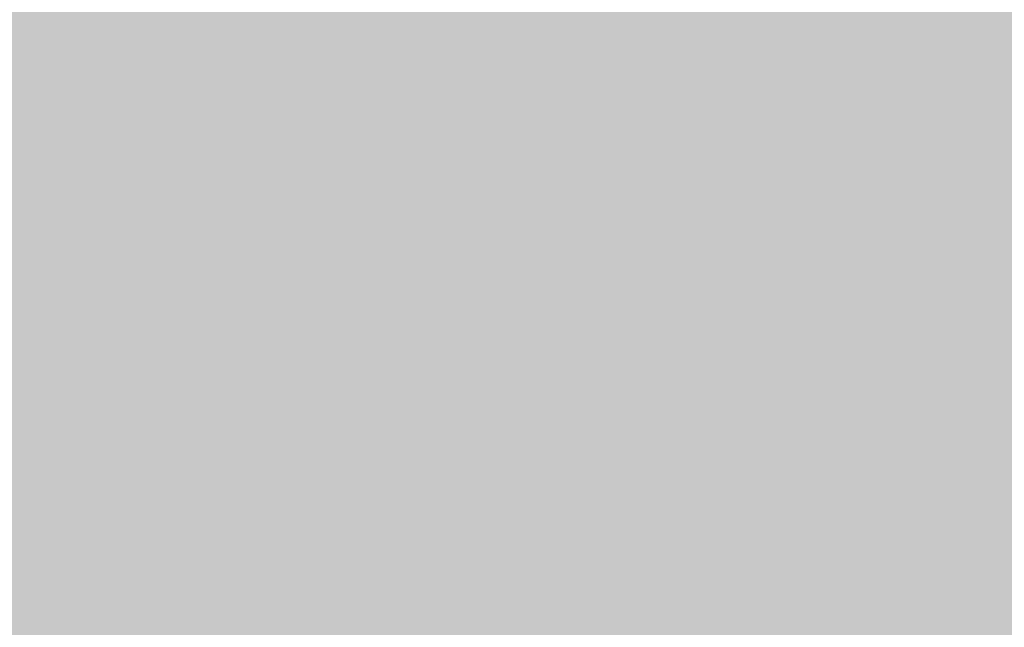
# Model space of a CAD drawing. Units: millimetres. Extents: x 0 to 2267, y 0 to 1823.
# Tile 44 of 256: x 1593.7801 to 1594.2193, y 1226.1145 to 1226.3857. Entities that reach past the tile are written whole.
import ezdxf

# ---------------------------------------------------------------- set-up
doc = ezdxf.new("R2010")
doc.units = ezdxf.units.MM
doc.header["$MEASUREMENT"] = 0
doc.layers.add('M-HATC', color=252, linetype='Continuous', lineweight=18)

msp = doc.modelspace()

# ---------------------------------------------------------------- hatches: boundary and pattern name
at = {"layer": 'M-HATC'}
h = msp.add_hatch(color=256, dxfattribs=at)
h.dxf.hatch_style = 1
h.paths.add_polyline_path([(2055.77105, 1603.06204), (1381.08677, 1603.06204), (1381.08677, 1598.06204), (2055.77105, 1598.06204)])
h.paths.add_polyline_path([(2055.77105, 1598.06204), (1381.08677, 1598.06204), (1381.08677, 1593.06204), (2055.77105, 1593.06204)])
h.paths.add_polyline_path([(2051.30737, 1536.76088), (1385.55044, 1536.76088), (1385.55044, 1526.76088), (1387.55044, 1526.76088), (1388.53662, 1525.05276), (1385.33187, 1521.23348), (1385.33187, 1521.22256), (2050.25417, 1522.74913), (2048.32119, 1525.05276), (2049.30737, 1526.76088), (2051.30737, 1526.76088)])
edge = h.paths.add_edge_path()
edge.add_arc((1847.53451, 1379.14917), 135, 222.6030607, 222.8908505, ccw=False)
edge.add_line((1748.16629, 1287.76561), (1683.09212, 1287.76561))
edge.add_arc((1583.7239, 1379.14917), 135, 317.1091495, 317.3969393, ccw=False)
edge.add_arc((1678.9686, 1290.67067), 5, 222.89085, 317.10915, ccw=False)
edge.add_arc((1774.21331, 1379.14917), 135, 222.6030607, 222.8908505, ccw=False)
edge.add_line((1674.84509, 1287.76561), (1609.77092, 1287.76561))
edge.add_arc((1510.4027, 1379.14917), 135, 317.1091495, 317.3969393, ccw=False)
edge.add_arc((1605.6474, 1290.67067), 5, 222.89085, 317.10915, ccw=False)
edge.add_arc((1700.89211, 1379.14917), 135, 222.6030607, 222.8908505, ccw=False)
edge.add_line((1601.52388, 1287.76561), (1536.44972, 1287.76561))
edge.add_arc((1437.08149, 1379.14917), 135, 317.1091495, 317.3969393, ccw=False)
edge.add_arc((1532.3262, 1290.67067), 5, 222.89085, 317.10915, ccw=False)
edge.add_arc((1627.57091, 1379.14917), 135, 222.6030607, 222.8908505, ccw=False)
edge.add_line((1528.20268, 1287.76561), (1505.92891, 1287.76561))
edge.add_spline(control_points=[(1505.92891, 1287.76561), (1504.26224, 1287.76561), (1504.26224, 1282.76561), (1505.92891, 1282.76561)], knot_values=[0, 0, 0, 0, 5, 5, 5, 5], degree=3, periodic=0)
edge.add_line((1505.92891, 1282.76561), (1930.92891, 1282.76561))
edge.add_spline(control_points=[(1930.92891, 1282.76561), (1932.59557, 1282.76561), (1932.59557, 1287.76561), (1930.92891, 1287.76561)], knot_values=[0, 0, 0, 0, 5, 5, 5, 5], degree=3, periodic=0)
edge.add_line((1930.92891, 1287.76561), (1903.05573, 1287.76561))
edge.add_arc((1803.6875, 1379.14917), 135, 317.1091495, 317.3969393, ccw=False)
edge.add_arc((1898.93221, 1290.67067), 5, 222.89085, 317.10915, ccw=False)
edge.add_arc((1994.17691, 1379.14917), 135, 222.6030607, 222.8908505, ccw=False)
edge.add_line((1894.80869, 1287.76561), (1829.73452, 1287.76561))
edge.add_arc((1730.3663, 1379.14917), 135, 317.1091495, 317.3969393, ccw=False)
edge.add_arc((1825.61101, 1290.67067), 5, 222.89085, 317.10915, ccw=False)
edge.add_arc((1920.85571, 1379.14917), 135, 222.6030607, 222.8908505, ccw=False)
edge.add_line((1821.48749, 1287.76561), (1756.41332, 1287.76561))
edge.add_arc((1657.0451, 1379.14917), 135, 317.1091495, 317.3969393, ccw=False)
edge.add_arc((1752.28981, 1290.67067), 5, 222.89085, 317.10915, ccw=False)
edge = h.paths.add_edge_path()
edge.add_spline(control_points=[(1843.42891, 1227.24746), (1845.09557, 1227.24746), (1845.09557, 1232.24746), (1843.42891, 1232.24746)], knot_values=[0, 0, 0, 0, 5, 5, 5, 5], degree=3, periodic=0)
edge.add_line((1843.42891, 1232.24746), (1593.42891, 1232.24746))
edge.add_spline(control_points=[(1593.42891, 1232.24746), (1591.76224, 1232.24746), (1591.76224, 1227.24746), (1593.42891, 1227.24746)], knot_values=[0, 0, 0, 0, 5, 5, 5, 5], degree=3, periodic=0)
edge.add_line((1593.42891, 1227.24746), (1843.42891, 1227.24746))
h.paths.add_polyline_path([(1905.92891, 1127.41706), (1530.92891, 1127.41706, 0.414214), (1520.92891, 1117.41706), (1530.92891, 1117.41706), (1915.92891, 1117.41706, 0.414214)])
edge = h.paths.add_edge_path()
edge.add_arc((1397.08577, 1498.40775), 12.72993, 90.782146, 190.878706, ccw=False)
edge.add_line((1396.912, 1511.13649), (1428.00968, 1511.34875))
edge.add_line((1428.00968, 1511.34875), (1433.00968, 1511.34875))
edge.add_line((1433.00968, 1511.34875), (1434.439, 1511.34875))
edge.add_arc((1419.474, 1498.08041), 20, 41.560995, 74.082109)
edge.add_line((1424.95919, 1517.31353), (1399.93509, 1517.25608))
edge.add_spline(control_points=[(1399.93074, 1517.25607), (1399.88398, 1517.21312), (1399.8328, 1517.16893), (1399.77741, 1517.1236)], knot_values=[11.567499, 11.567499, 11.567499, 11.567499, 11.814249, 11.814249, 11.814249, 11.814249], degree=3, periodic=0)
edge.add_spline(control_points=[(1399.63279, 1517.00986), (1399.58305, 1516.97214), (1399.53072, 1516.93375), (1399.47591, 1516.89474)], knot_values=[11.167718, 11.167718, 11.167718, 11.167718, 11.365188, 11.365188, 11.365188, 11.365188], degree=3, periodic=0)
edge.add_spline(control_points=[(1399.33981, 1516.80007), (1399.15144, 1516.67185), (1398.93836, 1516.5377), (1398.70404, 1516.39942)], knot_values=[10.376405, 10.376405, 10.376405, 10.376405, 11.00994, 11.00994, 11.00994, 11.00994], degree=3, periodic=0)
edge.add_spline(control_points=[(1398.65716, 1516.37187), (1398.57885, 1516.32602), (1398.49825, 1516.27974), (1398.41549, 1516.23309)], knot_values=[10.125175, 10.125175, 10.125175, 10.125175, 10.334406, 10.334406, 10.334406, 10.334406], degree=3, periodic=0)
edge.add_spline(control_points=[(1398.26422, 1516.14874), (1398.19595, 1516.11107), (1398.12634, 1516.07319), (1398.05546, 1516.03513)], knot_values=[9.832246, 9.832246, 9.832246, 9.832246, 9.999658, 9.999658, 9.999658, 9.999658], degree=3, periodic=0)
edge.add_spline(control_points=[(1397.9987, 1516.00476), (1397.73115, 1515.86211), (1397.44602, 1515.71707), (1397.14664, 1515.57138)], knot_values=[9.161808, 9.161808, 9.161808, 9.161808, 9.787769, 9.787769, 9.787769, 9.787769], degree=3, periodic=0)
edge.add_spline(control_points=[(1397.14664, 1515.57138), (1396.84182, 1515.42305), (1396.52223, 1515.27404), (1396.1914, 1515.12621)], knot_values=[8.524455, 8.524455, 8.524455, 8.524455, 9.161808, 9.161808, 9.161808, 9.161808], degree=3, periodic=0)
edge.add_spline(control_points=[(1396.07771, 1515.07565), (1395.98538, 1515.03478), (1395.89222, 1514.99402), (1395.7983, 1514.9534)], knot_values=[8.275193, 8.275193, 8.275193, 8.275193, 8.451726, 8.451726, 8.451726, 8.451726], degree=3, periodic=0)
edge.add_spline(control_points=[(1395.60184, 1514.86912), (1395.49975, 1514.82568), (1395.39685, 1514.78244), (1395.29322, 1514.73944)], knot_values=[7.962917, 7.962917, 7.962917, 7.962917, 8.152764, 8.152764, 8.152764, 8.152764], degree=3, periodic=0)
edge.add_spline(control_points=[(1395.21158, 1514.70568), (1394.82779, 1514.5475), (1394.43452, 1514.39287), (1394.03645, 1514.24422)], knot_values=[7.21254, 7.21254, 7.21254, 7.21254, 7.913148, 7.913148, 7.913148, 7.913148], degree=3, periodic=0)
edge.add_spline(control_points=[(1394.03645, 1514.24422), (1393.70758, 1514.12142), (1393.37544, 1514.0027), (1393.04267, 1513.88945)], knot_values=[6.633733, 6.633733, 6.633733, 6.633733, 7.21254, 7.21254, 7.21254, 7.21254], degree=3, periodic=0)
edge.add_spline(control_points=[(1392.82142, 1513.81499), (1392.71978, 1513.78118), (1392.61815, 1513.74791), (1392.51658, 1513.71521)], knot_values=[6.328796, 6.328796, 6.328796, 6.328796, 6.505493, 6.505493, 6.505493, 6.505493], degree=3, periodic=0)
edge.add_spline(control_points=[(1392.51658, 1513.71521), (1392.31873, 1513.65151), (1392.12116, 1513.59001), (1391.92441, 1513.53098)], knot_values=[5.984605, 5.984605, 5.984605, 5.984605, 6.328796, 6.328796, 6.328796, 6.328796], degree=3, periodic=0)
edge.add_spline(control_points=[(1391.79155, 1513.49146), (1391.31215, 1513.35011), (1390.83842, 1513.22392), (1390.37844, 1513.11711)], knot_values=[5.066697, 5.066697, 5.066697, 5.066697, 5.907055, 5.907055, 5.907055, 5.907055], degree=3, periodic=0)
edge.add_spline(control_points=[(1390.37844, 1513.11711), (1390.17973, 1513.07097), (1389.98359, 1513.02845), (1389.79067, 1512.98988)], knot_values=[4.70367, 4.70367, 4.70367, 4.70367, 5.066695, 5.066695, 5.066695, 5.066695], degree=3, periodic=0)
edge.add_spline(control_points=[(1389.42203, 1512.92036), (1389.24588, 1512.88922), (1389.0729, 1512.86172), (1388.90364, 1512.83814)], knot_values=[4.130571, 4.130571, 4.130571, 4.130571, 4.469816, 4.469816, 4.469816, 4.469816], degree=3, periodic=0)
edge.add_spline(control_points=[(1388.90364, 1512.83814), (1388.59103, 1512.7946), (1388.29108, 1512.76444), (1388.00714, 1512.74941)], knot_values=[3.504031, 3.504031, 3.504031, 3.504031, 4.130571, 4.130571, 4.130571, 4.130571], degree=3, periodic=0)
edge.add_spline(control_points=[(1387.9356, 1512.74593), (1387.85378, 1512.74231), (1387.77334, 1512.73997), (1387.69435, 1512.73898)], knot_values=[3.268866, 3.268866, 3.268866, 3.268866, 3.451164, 3.451164, 3.451164, 3.451164], degree=3, periodic=0)
edge.add_spline(control_points=[(1387.33512, 1512.74426), (1387.20757, 1512.74991), (1387.08472, 1512.7597), (1386.96699, 1512.77385)], knot_values=[2.670686, 2.670686, 2.670686, 2.670686, 2.984, 2.984, 2.984, 2.984], degree=3, periodic=0)
edge.add_spline(control_points=[(1386.83274, 1512.79225), (1386.82093, 1512.79407), (1386.80917, 1512.79594), (1386.79747, 1512.79787)], knot_values=[2.516981, 2.516981, 2.516981, 2.516981, 2.549528, 2.549528, 2.549528, 2.549528], degree=3, periodic=0)
edge.add_spline(control_points=[(1386.45257, 1512.87348), (1386.42573, 1512.88105), (1386.39931, 1512.88895), (1386.3733, 1512.89719)], knot_values=[2.095869, 2.095869, 2.095869, 2.095869, 2.17941, 2.17941, 2.17941, 2.17941], degree=3, periodic=0)
edge.add_spline(control_points=[(1386.06911, 1513.01889), (1386.06338, 1513.02174), (1386.05768, 1513.02463), (1386.05201, 1513.02753)], knot_values=[1.72453, 1.72453, 1.72453, 1.72453, 1.745933, 1.745933, 1.745933, 1.745933], degree=3, periodic=0)
edge.add_arc((1399.474, 1498.08041), 20, 131.824322, 180)
edge.add_arc((1630.33362, 1505.54843), 250.97076, 181.7051759, 236.427975)
edge.add_arc((1605.33992, 1483.30441), 218.7822, 238.660829, 243.3496099)
edge.add_arc((1647.09105, 1510.35917), 262.89859, 183.1298361, 237.8534422, ccw=False)
h.paths.add_polyline_path([(1406.53685, 1391.96444, 0.149382), (1491.55061, 1296.44177, -0.129517)], flags=17)
edge = h.paths.add_edge_path()
edge.add_arc((2037.38381, 1498.08041), 20, 0, 48.265868)
edge.add_spline(control_points=[(2050.69731, 1513.00525), (2050.65121, 1512.98471), (2050.60338, 1512.96554), (2050.55388, 1512.94771)], knot_values=[1.835652, 1.835652, 1.835652, 1.835652, 2.000781, 2.000781, 2.000781, 2.000781], degree=3, periodic=0)
edge.add_spline(control_points=[(2050.46156, 1512.91661), (2050.479, 1512.9221), (2050.49625, 1512.92774), (2050.51332, 1512.93353)], knot_values=[2.045477, 2.045477, 2.045477, 2.045477, 2.101389, 2.101389, 2.101389, 2.101389], degree=3, periodic=0)
edge.add_spline(control_points=[(2050.12896, 1512.83416), (2050.19843, 1512.84734), (2050.26573, 1512.86233), (2050.33075, 1512.87919)], knot_values=[2.237629, 2.237629, 2.237629, 2.237629, 2.435841, 2.435841, 2.435841, 2.435841], degree=3, periodic=0)
edge.add_spline(control_points=[(2050.09463, 1512.82783), (2050.10613, 1512.82989), (2050.11757, 1512.832), (2050.12896, 1512.83416)], knot_values=[2.435841, 2.435841, 2.435841, 2.435841, 2.468321, 2.468321, 2.468321, 2.468321], degree=3, periodic=0)
edge.add_spline(control_points=[(2049.78433, 1512.78511), (2049.85521, 1512.79219), (2049.92435, 1512.80077), (2049.99166, 1512.81088)], knot_values=[2.563852, 2.563852, 2.563852, 2.563852, 2.748541, 2.748541, 2.748541, 2.748541], degree=3, periodic=0)
edge.add_spline(control_points=[(2049.4052, 1512.76169), (2049.5364, 1512.76526), (2049.66292, 1512.77299), (2049.78433, 1512.78511)], knot_values=[2.748541, 2.748541, 2.748541, 2.748541, 3.064882, 3.064882, 3.064882, 3.064882], degree=3, periodic=0)
edge.add_spline(control_points=[(2049.16976, 1512.75968), (2049.23364, 1512.7591), (2049.29654, 1512.7594), (2049.35844, 1512.7606)], knot_values=[3.102309, 3.102309, 3.102309, 3.102309, 3.2503, 3.2503, 3.2503, 3.2503], degree=3, periodic=0)
edge.add_spline(control_points=[(2048.85727, 1512.76911), (2048.96378, 1512.76378), (2049.068, 1512.76061), (2049.16976, 1512.75968)], knot_values=[3.2503, 3.2503, 3.2503, 3.2503, 3.486069, 3.486069, 3.486069, 3.486069], degree=3, periodic=0)
edge.add_spline(control_points=[(2048.69241, 1512.77892), (2048.3729, 1512.80093), (2048.0345, 1512.84106), (2047.68175, 1512.89697)], knot_values=[3.606429, 3.606429, 3.606429, 3.606429, 4.2989, 4.2989, 4.2989, 4.2989], degree=3, periodic=0)
edge.add_spline(control_points=[(2047.68175, 1512.89697), (2047.5458, 1512.91852), (2047.40772, 1512.94241), (2047.26776, 1512.96851)], knot_values=[4.2989, 4.2989, 4.2989, 4.2989, 4.565769, 4.565769, 4.565769, 4.565769], degree=3, periodic=0)
edge.add_spline(control_points=[(2047.26776, 1512.96851), (2047.14494, 1512.99141), (2047.02067, 1513.01601), (2046.89514, 1513.04223)], knot_values=[4.565769, 4.565769, 4.565769, 4.565769, 4.799971, 4.799971, 4.799971, 4.799971], degree=3, periodic=0)
edge.add_spline(control_points=[(2046.89514, 1513.04223), (2046.52865, 1513.11875), (2046.15135, 1513.20899), (2045.7676, 1513.31068)], knot_values=[4.799971, 4.799971, 4.799971, 4.799971, 5.483718, 5.483718, 5.483718, 5.483718], degree=3, periodic=0)
edge.add_spline(control_points=[(2045.7676, 1513.31068), (2045.3724, 1513.41539), (2044.97036, 1513.53225), (2044.56625, 1513.65876)], knot_values=[5.483718, 5.483718, 5.483718, 5.483718, 6.187866, 6.187866, 6.187866, 6.187866], degree=3, periodic=0)
edge.add_spline(control_points=[(2044.56625, 1513.65876), (2044.41491, 1513.70614), (2044.26329, 1513.75487), (2044.11163, 1513.80482)], knot_values=[6.187866, 6.187866, 6.187866, 6.187866, 6.451551, 6.451551, 6.451551, 6.451551], degree=3, periodic=0)
edge.add_spline(control_points=[(2044.11163, 1513.80482), (2043.99666, 1513.84269), (2043.88167, 1513.88126), (2043.76676, 1513.92048)], knot_values=[6.451551, 6.451551, 6.451551, 6.451551, 6.651434, 6.651434, 6.651434, 6.651434], degree=3, periodic=0)
edge.add_spline(control_points=[(2043.76676, 1513.92048), (2043.37157, 1514.05536), (2042.97738, 1514.19789), (2042.58863, 1514.34575)], knot_values=[6.651434, 6.651434, 6.651434, 6.651434, 7.338879, 7.338879, 7.338879, 7.338879], degree=3, periodic=0)
edge.add_spline(control_points=[(2042.58863, 1514.34575), (2042.16431, 1514.50715), (2041.74647, 1514.67491), (2041.34086, 1514.84603)], knot_values=[7.338879, 7.338879, 7.338879, 7.338879, 8.089209, 8.089209, 8.089209, 8.089209], degree=3, periodic=0)
edge.add_spline(control_points=[(2041.34086, 1514.84603), (2041.1028, 1514.94647), (2040.86896, 1515.04806), (2040.64049, 1515.1502)], knot_values=[8.089209, 8.089209, 8.089209, 8.089209, 8.529587, 8.529587, 8.529587, 8.529587], degree=3, periodic=0)
edge.add_spline(control_points=[(2040.50999, 1515.20887), (2040.08238, 1515.40218), (2039.67475, 1515.59705), (2039.29495, 1515.78939)], knot_values=[8.613818, 8.613818, 8.613818, 8.613818, 9.44571, 9.44571, 9.44571, 9.44571], degree=3, periodic=0)
edge.add_spline(control_points=[(2039.29495, 1515.78939), (2039.0618, 1515.90746), (2038.83914, 1516.02458), (2038.62878, 1516.1398)], knot_values=[9.44571, 9.44571, 9.44571, 9.44571, 9.956404, 9.956404, 9.956404, 9.956404], degree=3, periodic=0)
edge.add_spline(control_points=[(2038.62878, 1516.1398), (2038.51874, 1516.20007), (2038.41207, 1516.25982), (2038.30903, 1516.31891)], knot_values=[9.956404, 9.956404, 9.956404, 9.956404, 10.223542, 10.223542, 10.223542, 10.223542], degree=3, periodic=0)
edge.add_spline(control_points=[(2038.30903, 1516.31891), (2038.21377, 1516.37354), (2038.12161, 1516.42762), (2038.03275, 1516.48102)], knot_values=[10.223542, 10.223542, 10.223542, 10.223542, 10.47051, 10.47051, 10.47051, 10.47051], degree=3, periodic=0)
edge.add_spline(control_points=[(2038.03275, 1516.48102), (2037.78552, 1516.62961), (2037.56388, 1516.77304), (2037.37225, 1516.909)], knot_values=[10.47051, 10.47051, 10.47051, 10.47051, 11.15767, 11.15767, 11.15767, 11.15767], degree=3, periodic=0)
edge.add_spline(control_points=[(2037.37225, 1516.909), (2037.27893, 1516.9752), (2037.19274, 1517.03963), (2037.11417, 1517.10203)], knot_values=[11.15767, 11.15767, 11.15767, 11.15767, 11.49227, 11.49227, 11.49227, 11.49227], degree=3, periodic=0)
edge.add_spline(control_points=[(2036.85638, 1517.32585), (2036.91481, 1517.26923), (2036.98143, 1517.21027), (2037.05573, 1517.14922)], knot_values=[11.577341, 11.577341, 11.577341, 11.577341, 11.91035, 11.91035, 11.91035, 11.91035], degree=3, periodic=0)
edge.add_spline(control_points=[(2036.80739, 1517.37475), (2036.82301, 1517.35865), (2036.83935, 1517.34235), (2036.85638, 1517.32585)], knot_values=[11.91035, 11.91035, 11.91035, 11.91035, 12.007402, 12.007402, 12.007402, 12.007402], degree=3, periodic=0)
edge.add_spline(control_points=[(2036.70167, 1517.494), (2036.71042, 1517.48299), (2036.71958, 1517.47185), (2036.72913, 1517.4606)], knot_values=[12.184155, 12.184155, 12.184155, 12.184155, 12.255409, 12.255409, 12.255409, 12.255409], degree=3, periodic=0)
edge.add_spline(control_points=[(2036.6159, 1517.6205), (2036.61998, 1517.61304), (2036.6243, 1517.6055), (2036.62885, 1517.59789)], knot_values=[12.487913, 12.487913, 12.487913, 12.487913, 12.541035, 12.541035, 12.541035, 12.541035], degree=3, periodic=0)
edge.add_spline(control_points=[(2036.56349, 1517.78599), (2036.56372, 1517.77936), (2036.56423, 1517.77264), (2036.56502, 1517.76582)], knot_values=[12.911761, 12.911761, 12.911761, 12.911761, 12.968286, 12.968286, 12.968286, 12.968286], degree=3, periodic=0)
edge.add_spline(control_points=[(2036.61663, 1517.93042), (2036.61248, 1517.92586), (2036.60857, 1517.92121), (2036.60491, 1517.91648)], knot_values=[13.382527, 13.382527, 13.382527, 13.382527, 13.433791, 13.433791, 13.433791, 13.433791], degree=3, periodic=0)
edge.add_spline(control_points=[(2036.74902, 1518.01695), (2036.73613, 1518.0116), (2036.72393, 1518.00601), (2036.71242, 1518.00018)], knot_values=[13.726299, 13.726299, 13.726299, 13.726299, 13.809928, 13.809928, 13.809928, 13.809928], degree=3, periodic=0)
edge.add_spline(control_points=[(2036.86043, 1518.05285), (2036.83863, 1518.04743), (2036.81809, 1518.04156), (2036.79879, 1518.03526)], knot_values=[13.910887, 13.910887, 13.910887, 13.910887, 14.02153, 14.02153, 14.02153, 14.02153], degree=3, periodic=0)
edge.add_line((2036.96387, 1518.08041), (2032.38381, 1518.08041))
edge.add_line((2032.38381, 1518.08041), (2027.38381, 1518.08041))
edge.add_line((2027.38381, 1518.08041), (2022.38381, 1518.08041))
edge.add_line((2022.38381, 1518.08041), (2017.38381, 1518.08041))
edge.add_arc((2017.38381, 1498.08041), 20, 90, 138.439005)
edge.add_line((2002.41881, 1511.34875), (2003.84813, 1511.34875))
edge.add_line((2003.84813, 1511.34875), (2008.84813, 1511.34875))
edge.add_line((2008.84813, 1511.34875), (2039.77204, 1511.13768))
edge.add_arc((2039.77204, 1498.40775), 12.72993, -10.878706, 90, ccw=False)
edge.add_arc((1789.76676, 1510.35917), 262.89859, 302.1465578, 356.8701639, ccw=False)
edge.add_arc((1831.51789, 1483.30441), 218.7822, 296.6503901, 301.339171)
edge.add_arc((1806.52419, 1505.54843), 250.97076, 303.572025, 358.2948241)
h.paths.add_polyline_path([(2030.32096, 1391.96444, -0.129517), (1945.3072, 1296.44177, 0.149382)], flags=17)
edge = h.paths.add_edge_path()
edge.add_spline(control_points=[(2037.2464, 1518.08209), (2037.28977, 1518.08098), (2037.33555, 1518.08041), (2037.3838, 1518.08041)], knot_values=[0.000012, 0.000012, 0.000012, 0.000012, 0.144754, 0.144754, 0.144754, 0.144754], degree=3, periodic=0)
edge.add_line((2037.33571, 1518.08041), (2037.00963, 1518.08041))
edge.add_spline(control_points=[(2037.00963, 1518.08041), (2036.98217, 1518.07678), (2036.95605, 1518.07266), (2036.93124, 1518.06808)], knot_values=[14.13465, 14.13465, 14.13465, 14.13465, 14.247197, 14.247197, 14.247197, 14.247197], degree=3, periodic=0)
edge.add_spline(control_points=[(2036.93124, 1518.06808), (2036.92764, 1518.06741), (2036.92407, 1518.06674), (2036.92053, 1518.06605)], knot_values=[14.118315, 14.118315, 14.118315, 14.118315, 14.13465, 14.13465, 14.13465, 14.13465], degree=3, periodic=0)
edge.add_spline(control_points=[(2036.92053, 1518.06605), (2036.9118, 1518.06436), (2036.90323, 1518.06262), (2036.89484, 1518.06081)], knot_values=[14.078086, 14.078086, 14.078086, 14.078086, 14.118315, 14.118315, 14.118315, 14.118315], degree=3, periodic=0)
edge.add_spline(control_points=[(2036.89484, 1518.06081), (2036.88304, 1518.05827), (2036.87157, 1518.05562), (2036.86043, 1518.05285)], knot_values=[14.02153, 14.02153, 14.02153, 14.02153, 14.078086, 14.078086, 14.078086, 14.078086], degree=3, periodic=0)
edge.add_spline(control_points=[(2036.86043, 1518.05285), (2036.83863, 1518.04743), (2036.81809, 1518.04156), (2036.79879, 1518.03526)], knot_values=[13.910887, 13.910887, 13.910887, 13.910887, 14.02153, 14.02153, 14.02153, 14.02153], degree=3, periodic=0)
edge.add_spline(control_points=[(2036.79879, 1518.03526), (2036.79809, 1518.03504), (2036.7974, 1518.03481), (2036.79671, 1518.03458)], knot_values=[13.906906, 13.906906, 13.906906, 13.906906, 13.910887, 13.910887, 13.910887, 13.910887], degree=3, periodic=0)
edge.add_spline(control_points=[(2036.79671, 1518.03458), (2036.78819, 1518.03178), (2036.77991, 1518.02888), (2036.77187, 1518.02591)], knot_values=[13.857826, 13.857826, 13.857826, 13.857826, 13.906906, 13.906906, 13.906906, 13.906906], degree=3, periodic=0)
edge.add_spline(control_points=[(2036.77187, 1518.02591), (2036.76402, 1518.023), (2036.75641, 1518.02002), (2036.74902, 1518.01695)], knot_values=[13.809928, 13.809928, 13.809928, 13.809928, 13.857826, 13.857826, 13.857826, 13.857826], degree=3, periodic=0)
edge.add_spline(control_points=[(2036.74902, 1518.01695), (2036.73613, 1518.0116), (2036.72393, 1518.00601), (2036.71242, 1518.00018)], knot_values=[13.726299, 13.726299, 13.726299, 13.726299, 13.809928, 13.809928, 13.809928, 13.809928], degree=3, periodic=0)
edge.add_spline(control_points=[(2036.71242, 1518.00018), (2036.71211, 1518.00002), (2036.71179, 1517.99986), (2036.71147, 1517.99969)], knot_values=[13.723993, 13.723993, 13.723993, 13.723993, 13.726299, 13.726299, 13.726299, 13.726299], degree=3, periodic=0)
edge.add_spline(control_points=[(2036.71147, 1517.99969), (2036.70634, 1517.99708), (2036.70134, 1517.99441), (2036.69648, 1517.9917)], knot_values=[13.686536, 13.686536, 13.686536, 13.686536, 13.723993, 13.723993, 13.723993, 13.723993], degree=3, periodic=0)
edge.add_spline(control_points=[(2036.69648, 1517.9917), (2036.6919, 1517.98914), (2036.68744, 1517.98654), (2036.6831, 1517.9839)], knot_values=[13.651251, 13.651251, 13.651251, 13.651251, 13.686536, 13.686536, 13.686536, 13.686536], degree=3, periodic=0)
edge.add_spline(control_points=[(2036.6831, 1517.9839), (2036.67641, 1517.97983), (2036.67001, 1517.97566), (2036.6639, 1517.97139)], knot_values=[13.596804, 13.596804, 13.596804, 13.596804, 13.651251, 13.651251, 13.651251, 13.651251], degree=3, periodic=0)
edge.add_spline(control_points=[(2036.6639, 1517.97139), (2036.66358, 1517.97117), (2036.66326, 1517.97094), (2036.66294, 1517.97072)], knot_values=[13.593956, 13.593956, 13.593956, 13.593956, 13.596804, 13.596804, 13.596804, 13.596804], degree=3, periodic=0)
edge.add_spline(control_points=[(2036.66294, 1517.97072), (2036.6603, 1517.96886), (2036.65771, 1517.96698), (2036.65518, 1517.96509)], knot_values=[13.570322, 13.570322, 13.570322, 13.570322, 13.593956, 13.593956, 13.593956, 13.593956], degree=3, periodic=0)
edge.add_spline(control_points=[(2036.65518, 1517.96509), (2036.65251, 1517.9631), (2036.64991, 1517.96108), (2036.64737, 1517.95905)], knot_values=[13.545477, 13.545477, 13.545477, 13.545477, 13.570322, 13.570322, 13.570322, 13.570322], degree=3, periodic=0)
edge.add_spline(control_points=[(2036.64737, 1517.95905), (2036.64721, 1517.95892), (2036.64705, 1517.9588), (2036.64689, 1517.95867)], knot_values=[13.543931, 13.543931, 13.543931, 13.543931, 13.545477, 13.545477, 13.545477, 13.545477], degree=3, periodic=0)
edge.add_spline(control_points=[(2036.64689, 1517.95867), (2036.64121, 1517.95411), (2036.63582, 1517.94945), (2036.63073, 1517.94468)], knot_values=[13.488237, 13.488237, 13.488237, 13.488237, 13.543931, 13.543931, 13.543931, 13.543931], degree=3, periodic=0)
edge.add_spline(control_points=[(2036.63073, 1517.94468), (2036.62817, 1517.94229), (2036.62569, 1517.93988), (2036.62329, 1517.93744)], knot_values=[13.460307, 13.460307, 13.460307, 13.460307, 13.488237, 13.488237, 13.488237, 13.488237], degree=3, periodic=0)
edge.add_spline(control_points=[(2036.62329, 1517.93744), (2036.62151, 1517.93564), (2036.61978, 1517.93383), (2036.61809, 1517.932)], knot_values=[13.439712, 13.439712, 13.439712, 13.439712, 13.460307, 13.460307, 13.460307, 13.460307], degree=3, periodic=0)
edge.add_spline(control_points=[(2036.61809, 1517.932), (2036.6176, 1517.93147), (2036.61711, 1517.93095), (2036.61663, 1517.93042)], knot_values=[13.433791, 13.433791, 13.433791, 13.433791, 13.439712, 13.439712, 13.439712, 13.439712], degree=3, periodic=0)
edge.add_spline(control_points=[(2036.61663, 1517.93042), (2036.61248, 1517.92586), (2036.60857, 1517.92121), (2036.60491, 1517.91648)], knot_values=[13.382527, 13.382527, 13.382527, 13.382527, 13.433791, 13.433791, 13.433791, 13.433791], degree=3, periodic=0)
edge.add_spline(control_points=[(2036.60491, 1517.91648), (2036.60258, 1517.91347), (2036.60036, 1517.91044), (2036.59824, 1517.90737)], knot_values=[13.350017, 13.350017, 13.350017, 13.350017, 13.382527, 13.382527, 13.382527, 13.382527], degree=3, periodic=0)
edge.add_spline(control_points=[(2036.59824, 1517.90737), (2036.59718, 1517.90585), (2036.59616, 1517.90433), (2036.59515, 1517.90279)], knot_values=[13.333922, 13.333922, 13.333922, 13.333922, 13.350017, 13.350017, 13.350017, 13.350017], degree=3, periodic=0)
edge.add_spline(control_points=[(2036.59515, 1517.90279), (2036.59452, 1517.90183), (2036.5939, 1517.90086), (2036.59329, 1517.89989)], knot_values=[13.323828, 13.323828, 13.323828, 13.323828, 13.333922, 13.333922, 13.333922, 13.333922], degree=3, periodic=0)
edge.add_spline(control_points=[(2036.59329, 1517.89989), (2036.59049, 1517.89545), (2036.5879, 1517.89094), (2036.5855, 1517.88637)], knot_values=[13.277545, 13.277545, 13.277545, 13.277545, 13.323828, 13.323828, 13.323828, 13.323828], degree=3, periodic=0)
edge.add_spline(control_points=[(2036.5855, 1517.88637), (2036.58355, 1517.88267), (2036.58174, 1517.87892), (2036.58006, 1517.87513)], knot_values=[13.240119, 13.240119, 13.240119, 13.240119, 13.277545, 13.277545, 13.277545, 13.277545], degree=3, periodic=0)
edge.add_spline(control_points=[(2036.58006, 1517.87513), (2036.57952, 1517.87393), (2036.579, 1517.87272), (2036.57849, 1517.87151)], knot_values=[13.228211, 13.228211, 13.228211, 13.228211, 13.240119, 13.240119, 13.240119, 13.240119], degree=3, periodic=0)
edge.add_spline(control_points=[(2036.57849, 1517.87151), (2036.57796, 1517.87023), (2036.57744, 1517.86896), (2036.57693, 1517.86767)], knot_values=[13.215717, 13.215717, 13.215717, 13.215717, 13.228211, 13.228211, 13.228211, 13.228211], degree=3, periodic=0)
edge.add_spline(control_points=[(2036.57693, 1517.86767), (2036.57548, 1517.86399), (2036.57414, 1517.86027), (2036.57293, 1517.85651)], knot_values=[13.179847, 13.179847, 13.179847, 13.179847, 13.215717, 13.215717, 13.215717, 13.215717], degree=3, periodic=0)
edge.add_spline(control_points=[(2036.57293, 1517.85651), (2036.5713, 1517.8515), (2036.56989, 1517.84641), (2036.56868, 1517.84126)], knot_values=[13.132017, 13.132017, 13.132017, 13.132017, 13.179847, 13.179847, 13.179847, 13.179847], degree=3, periodic=0)
edge.add_spline(control_points=[(2036.56868, 1517.84126), (2036.56844, 1517.84023), (2036.56821, 1517.8392), (2036.56798, 1517.83817)], knot_values=[13.122482, 13.122482, 13.122482, 13.122482, 13.132017, 13.132017, 13.132017, 13.132017], degree=3, periodic=0)
edge.add_spline(control_points=[(2036.56798, 1517.83817), (2036.56758, 1517.83634), (2036.56721, 1517.8345), (2036.56687, 1517.83266)], knot_values=[13.105592, 13.105592, 13.105592, 13.105592, 13.122482, 13.122482, 13.122482, 13.122482], degree=3, periodic=0)
edge.add_spline(control_points=[(2036.56687, 1517.83266), (2036.56622, 1517.82921), (2036.56567, 1517.82574), (2036.5652, 1517.82223)], knot_values=[13.074063, 13.074063, 13.074063, 13.074063, 13.105592, 13.105592, 13.105592, 13.105592], degree=3, periodic=0)
edge.add_spline(control_points=[(2036.5652, 1517.82223), (2036.5652, 1517.82223), (2036.5652, 1517.82223), (2036.5652, 1517.82223)], knot_values=[13.074043, 13.074043, 13.074043, 13.074043, 13.074063, 13.074063, 13.074063, 13.074063], degree=3, periodic=0)
edge.add_spline(control_points=[(2036.5652, 1517.82223), (2036.56443, 1517.81643), (2036.5639, 1517.81055), (2036.56361, 1517.8046)], knot_values=[13.021884, 13.021884, 13.021884, 13.021884, 13.074043, 13.074043, 13.074043, 13.074043], degree=3, periodic=0)
edge.add_spline(control_points=[(2036.56361, 1517.8046), (2036.56358, 1517.80401), (2036.56356, 1517.80342), (2036.56353, 1517.80283)], knot_values=[13.01674, 13.01674, 13.01674, 13.01674, 13.021884, 13.021884, 13.021884, 13.021884], degree=3, periodic=0)
edge.add_spline(control_points=[(2036.56353, 1517.80283), (2036.56344, 1517.80051), (2036.56338, 1517.79817), (2036.56336, 1517.79582)], knot_values=[12.996438, 12.996438, 12.996438, 12.996438, 13.01674, 13.01674, 13.01674, 13.01674], degree=3, periodic=0)
edge.add_spline(control_points=[(2036.56336, 1517.79582), (2036.56334, 1517.79257), (2036.56338, 1517.78929), (2036.56349, 1517.78599)], knot_values=[12.968286, 12.968286, 12.968286, 12.968286, 12.996438, 12.996438, 12.996438, 12.996438], degree=3, periodic=0)
edge.add_spline(control_points=[(2036.56349, 1517.78599), (2036.56372, 1517.77936), (2036.56423, 1517.77264), (2036.56502, 1517.76582)], knot_values=[12.911761, 12.911761, 12.911761, 12.911761, 12.968286, 12.968286, 12.968286, 12.968286], degree=3, periodic=0)
edge.add_spline(control_points=[(2036.56502, 1517.76582), (2036.56503, 1517.76573), (2036.56504, 1517.76564), (2036.56505, 1517.76555)], knot_values=[12.911017, 12.911017, 12.911017, 12.911017, 12.911761, 12.911761, 12.911761, 12.911761], degree=3, periodic=0)
edge.add_spline(control_points=[(2036.56505, 1517.76555), (2036.56541, 1517.76245), (2036.56583, 1517.75933), (2036.56631, 1517.75619)], knot_values=[12.88528, 12.88528, 12.88528, 12.88528, 12.911017, 12.911017, 12.911017, 12.911017], degree=3, periodic=0)
edge.add_spline(control_points=[(2036.56631, 1517.75619), (2036.56673, 1517.75341), (2036.5672, 1517.75062), (2036.56771, 1517.74782)], knot_values=[12.862519, 12.862519, 12.862519, 12.862519, 12.88528, 12.88528, 12.88528, 12.88528], degree=3, periodic=0)
edge.add_spline(control_points=[(2036.56771, 1517.74782), (2036.56779, 1517.74737), (2036.56788, 1517.74692), (2036.56796, 1517.74647)], knot_values=[12.858885, 12.858885, 12.858885, 12.858885, 12.862519, 12.862519, 12.862519, 12.862519], degree=3, periodic=0)
edge.add_spline(control_points=[(2036.56796, 1517.74647), (2036.5692, 1517.73986), (2036.57069, 1517.73316), (2036.57243, 1517.72638)], knot_values=[12.8053, 12.8053, 12.8053, 12.8053, 12.858885, 12.858885, 12.858885, 12.858885], degree=3, periodic=0)
edge.add_spline(control_points=[(2036.57243, 1517.72638), (2036.5734, 1517.72257), (2036.57446, 1517.71874), (2036.57559, 1517.71488)], knot_values=[12.775176, 12.775176, 12.775176, 12.775176, 12.8053, 12.8053, 12.8053, 12.8053], degree=3, periodic=0)
edge.add_spline(control_points=[(2036.57559, 1517.71488), (2036.57628, 1517.71252), (2036.577, 1517.71015), (2036.57775, 1517.70778)], knot_values=[12.756759, 12.756759, 12.756759, 12.756759, 12.775176, 12.775176, 12.775176, 12.775176], degree=3, periodic=0)
edge.add_spline(control_points=[(2036.57775, 1517.70778), (2036.57808, 1517.70674), (2036.57841, 1517.7057), (2036.57875, 1517.70466)], knot_values=[12.748742, 12.748742, 12.748742, 12.748742, 12.756759, 12.756759, 12.756759, 12.756759], degree=3, periodic=0)
edge.add_spline(control_points=[(2036.57875, 1517.70466), (2036.58082, 1517.6983), (2036.58309, 1517.69187), (2036.58557, 1517.68537)], knot_values=[12.69959, 12.69959, 12.69959, 12.69959, 12.748742, 12.748742, 12.748742, 12.748742], degree=3, periodic=0)
edge.add_spline(control_points=[(2036.58557, 1517.68537), (2036.58762, 1517.68001), (2036.5898, 1517.6746), (2036.59213, 1517.66916)], knot_values=[12.659038, 12.659038, 12.659038, 12.659038, 12.69959, 12.69959, 12.69959, 12.69959], degree=3, periodic=0)
edge.add_spline(control_points=[(2036.59213, 1517.66916), (2036.59397, 1517.66482), (2036.59591, 1517.66047), (2036.59793, 1517.65608)], knot_values=[12.626806, 12.626806, 12.626806, 12.626806, 12.659038, 12.659038, 12.659038, 12.659038], degree=3, periodic=0)
edge.add_spline(control_points=[(2036.59793, 1517.65608), (2036.59839, 1517.65507), (2036.59886, 1517.65406), (2036.59934, 1517.65305)], knot_values=[12.619394, 12.619394, 12.619394, 12.619394, 12.626806, 12.626806, 12.626806, 12.626806], degree=3, periodic=0)
edge.add_spline(control_points=[(2036.59934, 1517.65305), (2036.60435, 1517.64236), (2036.60987, 1517.63151), (2036.61589, 1517.6205)], knot_values=[12.541039, 12.541039, 12.541039, 12.541039, 12.619394, 12.619394, 12.619394, 12.619394], degree=3, periodic=0)
edge.add_spline(control_points=[(2036.61589, 1517.6205), (2036.61589, 1517.6205), (2036.6159, 1517.6205), (2036.6159, 1517.6205)], knot_values=[12.541035, 12.541035, 12.541035, 12.541035, 12.541039, 12.541039, 12.541039, 12.541039], degree=3, periodic=0)
edge.add_spline(control_points=[(2036.6159, 1517.6205), (2036.61998, 1517.61304), (2036.6243, 1517.6055), (2036.62885, 1517.59789)], knot_values=[12.487913, 12.487913, 12.487913, 12.487913, 12.541035, 12.541035, 12.541035, 12.541035], degree=3, periodic=0)
edge.add_spline(control_points=[(2036.62885, 1517.59789), (2036.63261, 1517.5916), (2036.63653, 1517.58526), (2036.64061, 1517.57888)], knot_values=[12.443982, 12.443982, 12.443982, 12.443982, 12.487913, 12.487913, 12.487913, 12.487913], degree=3, periodic=0)
edge.add_spline(control_points=[(2036.64061, 1517.57888), (2036.64144, 1517.57757), (2036.64228, 1517.57626), (2036.64313, 1517.57495)], knot_values=[12.434996, 12.434996, 12.434996, 12.434996, 12.443982, 12.443982, 12.443982, 12.443982], degree=3, periodic=0)
edge.add_spline(control_points=[(2036.64313, 1517.57495), (2036.65306, 1517.55958), (2036.66389, 1517.54394), (2036.6756, 1517.52803)], knot_values=[12.329647, 12.329647, 12.329647, 12.329647, 12.434996, 12.434996, 12.434996, 12.434996], degree=3, periodic=0)
edge.add_spline(control_points=[(2036.6756, 1517.52803), (2036.68385, 1517.51682), (2036.69254, 1517.50548), (2036.70167, 1517.494)], knot_values=[12.255409, 12.255409, 12.255409, 12.255409, 12.329647, 12.329647, 12.329647, 12.329647], degree=3, periodic=0)
edge.add_spline(control_points=[(2036.70167, 1517.494), (2036.71042, 1517.48299), (2036.71958, 1517.47185), (2036.72913, 1517.4606)], knot_values=[12.184155, 12.184155, 12.184155, 12.184155, 12.255409, 12.255409, 12.255409, 12.255409], degree=3, periodic=0)
edge.add_spline(control_points=[(2036.72913, 1517.4606), (2036.74363, 1517.44352), (2036.75904, 1517.42617), (2036.77534, 1517.40855)], knot_values=[12.075961, 12.075961, 12.075961, 12.075961, 12.184155, 12.184155, 12.184155, 12.184155], degree=3, periodic=0)
edge.add_spline(control_points=[(2036.77534, 1517.40855), (2036.77631, 1517.4075), (2036.77729, 1517.40645), (2036.77827, 1517.40539)], knot_values=[12.069502, 12.069502, 12.069502, 12.069502, 12.075961, 12.075961, 12.075961, 12.075961], degree=3, periodic=0)
edge.add_spline(control_points=[(2036.77827, 1517.40539), (2036.78768, 1517.39526), (2036.79739, 1517.38505), (2036.80739, 1517.37475)], knot_values=[12.007402, 12.007402, 12.007402, 12.007402, 12.069502, 12.069502, 12.069502, 12.069502], degree=3, periodic=0)
edge.add_spline(control_points=[(2036.80739, 1517.37475), (2036.82301, 1517.35865), (2036.83935, 1517.34235), (2036.85638, 1517.32585)], knot_values=[11.91035, 11.91035, 11.91035, 11.91035, 12.007402, 12.007402, 12.007402, 12.007402], degree=3, periodic=0)
edge.add_spline(control_points=[(2036.85638, 1517.32585), (2036.91481, 1517.26923), (2036.98143, 1517.21027), (2037.05573, 1517.14922)], knot_values=[11.577341, 11.577341, 11.577341, 11.577341, 11.91035, 11.91035, 11.91035, 11.91035], degree=3, periodic=0)
edge.add_spline(control_points=[(2037.05573, 1517.14922), (2037.07471, 1517.13362), (2037.0942, 1517.11789), (2037.11417, 1517.10203)], knot_values=[11.49227, 11.49227, 11.49227, 11.49227, 11.577341, 11.577341, 11.577341, 11.577341], degree=3, periodic=0)
edge.add_spline(control_points=[(2037.11417, 1517.10203), (2037.19274, 1517.03963), (2037.27893, 1516.9752), (2037.37225, 1516.909)], knot_values=[11.15767, 11.15767, 11.15767, 11.15767, 11.49227, 11.49227, 11.49227, 11.49227], degree=3, periodic=0)
edge.add_spline(control_points=[(2037.37225, 1516.909), (2037.56388, 1516.77304), (2037.78552, 1516.62961), (2038.03275, 1516.48102)], knot_values=[10.47051, 10.47051, 10.47051, 10.47051, 11.15767, 11.15767, 11.15767, 11.15767], degree=3, periodic=0)
edge.add_spline(control_points=[(2038.03275, 1516.48102), (2038.12161, 1516.42762), (2038.21377, 1516.37354), (2038.30903, 1516.31891)], knot_values=[10.223542, 10.223542, 10.223542, 10.223542, 10.47051, 10.47051, 10.47051, 10.47051], degree=3, periodic=0)
edge.add_spline(control_points=[(2038.30903, 1516.31891), (2038.41207, 1516.25982), (2038.51874, 1516.20007), (2038.62878, 1516.1398)], knot_values=[9.956404, 9.956404, 9.956404, 9.956404, 10.223542, 10.223542, 10.223542, 10.223542], degree=3, periodic=0)
edge.add_spline(control_points=[(2038.62878, 1516.1398), (2038.83914, 1516.02458), (2039.0618, 1515.90746), (2039.29495, 1515.78939)], knot_values=[9.44571, 9.44571, 9.44571, 9.44571, 9.956404, 9.956404, 9.956404, 9.956404], degree=3, periodic=0)
edge.add_spline(control_points=[(2039.29495, 1515.78939), (2039.67475, 1515.59705), (2040.08238, 1515.40218), (2040.50999, 1515.20887)], knot_values=[8.613818, 8.613818, 8.613818, 8.613818, 9.44571, 9.44571, 9.44571, 9.44571], degree=3, periodic=0)
edge.add_spline(control_points=[(2040.50999, 1515.20887), (2040.55329, 1515.1893), (2040.59679, 1515.16974), (2040.64049, 1515.1502)], knot_values=[8.529587, 8.529587, 8.529587, 8.529587, 8.613818, 8.613818, 8.613818, 8.613818], degree=3, periodic=0)
edge.add_spline(control_points=[(2040.64049, 1515.1502), (2040.86896, 1515.04806), (2041.1028, 1514.94647), (2041.34086, 1514.84603)], knot_values=[8.089209, 8.089209, 8.089209, 8.089209, 8.529587, 8.529587, 8.529587, 8.529587], degree=3, periodic=0)
edge.add_spline(control_points=[(2041.34086, 1514.84603), (2041.74647, 1514.67491), (2042.16431, 1514.50715), (2042.58863, 1514.34575)], knot_values=[7.338879, 7.338879, 7.338879, 7.338879, 8.089209, 8.089209, 8.089209, 8.089209], degree=3, periodic=0)
edge.add_spline(control_points=[(2042.58863, 1514.34575), (2042.97738, 1514.19789), (2043.37157, 1514.05536), (2043.76676, 1513.92048)], knot_values=[6.651434, 6.651434, 6.651434, 6.651434, 7.338879, 7.338879, 7.338879, 7.338879], degree=3, periodic=0)
edge.add_spline(control_points=[(2043.76676, 1513.92048), (2043.88167, 1513.88126), (2043.99666, 1513.84269), (2044.11163, 1513.80482)], knot_values=[6.451551, 6.451551, 6.451551, 6.451551, 6.651434, 6.651434, 6.651434, 6.651434], degree=3, periodic=0)
edge.add_spline(control_points=[(2044.11163, 1513.80482), (2044.26329, 1513.75487), (2044.41491, 1513.70614), (2044.56625, 1513.65876)], knot_values=[6.187866, 6.187866, 6.187866, 6.187866, 6.451551, 6.451551, 6.451551, 6.451551], degree=3, periodic=0)
edge.add_spline(control_points=[(2044.56625, 1513.65876), (2044.97036, 1513.53225), (2045.3724, 1513.41539), (2045.7676, 1513.31068)], knot_values=[5.483718, 5.483718, 5.483718, 5.483718, 6.187866, 6.187866, 6.187866, 6.187866], degree=3, periodic=0)
edge.add_spline(control_points=[(2045.7676, 1513.31068), (2046.15135, 1513.20899), (2046.52865, 1513.11875), (2046.89514, 1513.04223)], knot_values=[4.799971, 4.799971, 4.799971, 4.799971, 5.483718, 5.483718, 5.483718, 5.483718], degree=3, periodic=0)
edge.add_spline(control_points=[(2046.89514, 1513.04223), (2047.02067, 1513.01601), (2047.14494, 1512.99141), (2047.26776, 1512.96851)], knot_values=[4.565769, 4.565769, 4.565769, 4.565769, 4.799971, 4.799971, 4.799971, 4.799971], degree=3, periodic=0)
edge.add_spline(control_points=[(2047.26776, 1512.96851), (2047.40772, 1512.94241), (2047.5458, 1512.91852), (2047.68175, 1512.89697)], knot_values=[4.2989, 4.2989, 4.2989, 4.2989, 4.565769, 4.565769, 4.565769, 4.565769], degree=3, periodic=0)
edge.add_spline(control_points=[(2047.68175, 1512.89697), (2048.0345, 1512.84106), (2048.3729, 1512.80093), (2048.69241, 1512.77892)], knot_values=[3.606429, 3.606429, 3.606429, 3.606429, 4.2989, 4.2989, 4.2989, 4.2989], degree=3, periodic=0)
edge.add_spline(control_points=[(2048.69241, 1512.77892), (2048.74794, 1512.7751), (2048.8029, 1512.77182), (2048.85727, 1512.76911)], knot_values=[3.486069, 3.486069, 3.486069, 3.486069, 3.606429, 3.606429, 3.606429, 3.606429], degree=3, periodic=0)
edge.add_spline(control_points=[(2048.85727, 1512.76911), (2048.96378, 1512.76378), (2049.068, 1512.76061), (2049.16976, 1512.75968)], knot_values=[3.2503, 3.2503, 3.2503, 3.2503, 3.486069, 3.486069, 3.486069, 3.486069], degree=3, periodic=0)
edge.add_spline(control_points=[(2049.16976, 1512.75968), (2049.23364, 1512.7591), (2049.29654, 1512.7594), (2049.35844, 1512.7606)], knot_values=[3.102309, 3.102309, 3.102309, 3.102309, 3.2503, 3.2503, 3.2503, 3.2503], degree=3, periodic=0)
edge.add_spline(control_points=[(2049.35844, 1512.7606), (2049.37409, 1512.76091), (2049.38968, 1512.76127), (2049.4052, 1512.76169)], knot_values=[3.064882, 3.064882, 3.064882, 3.064882, 3.102309, 3.102309, 3.102309, 3.102309], degree=3, periodic=0)
edge.add_spline(control_points=[(2049.4052, 1512.76169), (2049.5364, 1512.76526), (2049.66292, 1512.77299), (2049.78433, 1512.78511)], knot_values=[2.748541, 2.748541, 2.748541, 2.748541, 3.064882, 3.064882, 3.064882, 3.064882], degree=3, periodic=0)
edge.add_spline(control_points=[(2049.78433, 1512.78511), (2049.85521, 1512.79219), (2049.92435, 1512.80077), (2049.99166, 1512.81088)], knot_values=[2.563852, 2.563852, 2.563852, 2.563852, 2.748541, 2.748541, 2.748541, 2.748541], degree=3, periodic=0)
edge.add_spline(control_points=[(2049.99166, 1512.81088), (2050.02648, 1512.81612), (2050.0608, 1512.82177), (2050.09463, 1512.82783)], knot_values=[2.468321, 2.468321, 2.468321, 2.468321, 2.563852, 2.563852, 2.563852, 2.563852], degree=3, periodic=0)
edge.add_spline(control_points=[(2050.09463, 1512.82783), (2050.10613, 1512.82989), (2050.11757, 1512.832), (2050.12896, 1512.83416)], knot_values=[2.435841, 2.435841, 2.435841, 2.435841, 2.468321, 2.468321, 2.468321, 2.468321], degree=3, periodic=0)
edge.add_spline(control_points=[(2050.12896, 1512.83416), (2050.19843, 1512.84734), (2050.26573, 1512.86233), (2050.33075, 1512.87919)], knot_values=[2.237629, 2.237629, 2.237629, 2.237629, 2.435841, 2.435841, 2.435841, 2.435841], degree=3, periodic=0)
edge.add_spline(control_points=[(2050.33075, 1512.87919), (2050.37544, 1512.89077), (2050.41906, 1512.90324), (2050.46156, 1512.91661)], knot_values=[2.101389, 2.101389, 2.101389, 2.101389, 2.237629, 2.237629, 2.237629, 2.237629], degree=3, periodic=0)
edge.add_spline(control_points=[(2050.46156, 1512.91661), (2050.479, 1512.9221), (2050.49625, 1512.92774), (2050.51332, 1512.93353)], knot_values=[2.045477, 2.045477, 2.045477, 2.045477, 2.101389, 2.101389, 2.101389, 2.101389], degree=3, periodic=0)
edge.add_spline(control_points=[(2050.51332, 1512.93353), (2050.52696, 1512.93816), (2050.54048, 1512.94288), (2050.55388, 1512.94771)], knot_values=[2.000781, 2.000781, 2.000781, 2.000781, 2.045477, 2.045477, 2.045477, 2.045477], degree=3, periodic=0)
edge.add_spline(control_points=[(2050.55388, 1512.94771), (2050.60338, 1512.96554), (2050.65121, 1512.98471), (2050.69731, 1513.00525)], knot_values=[1.835652, 1.835652, 1.835652, 1.835652, 2.000781, 2.000781, 2.000781, 2.000781], degree=3, periodic=0)
edge.add_arc((2037.38381, 1498.08041), 20, 48.265868, 90.129934)
edge = h.paths.add_edge_path(flags=16)
edge.add_spline(control_points=[(1386.13885, 1512.98591), (1388.91997, 1511.73946), (1398.03873, 1515.51866), (1399.93074, 1517.25607)], knot_values=[1.831046, 1.831046, 1.831046, 1.831046, 11.814249, 11.814249, 11.814249, 11.814249], degree=3, periodic=0)
edge.add_line((1399.93074, 1517.25607), (1393.74348, 1517.24186))
edge.add_arc((1399.474, 1498.08041), 20, 106.650105, 131.817301)
h = msp.add_hatch(color=256, dxfattribs=at)
h.dxf.hatch_style = 1
h.paths.add_polyline_path([(2042.88863, 1580.17963), (2055.77105, 1593.06204), (1381.08677, 1593.06204), (1393.96918, 1580.17963), (1374.08597, 1560.29642), (2062.77184, 1560.29642)])
h.paths.add_polyline_path([(1843.42891, 1201.32971), (1843.42891, 1227.24746), (1593.42891, 1227.24746), (1593.42891, 1201.32971, -0.228274), (1574.59893, 1162.23457), (1530.92891, 1127.41706), (1905.92891, 1127.41706), (1862.25888, 1162.23457, -0.228274)])

doc.saveas('drawing.dxf')
